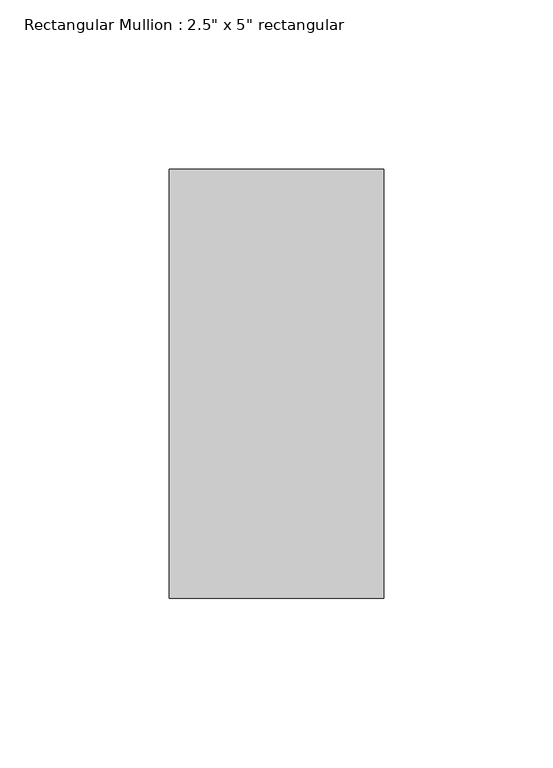
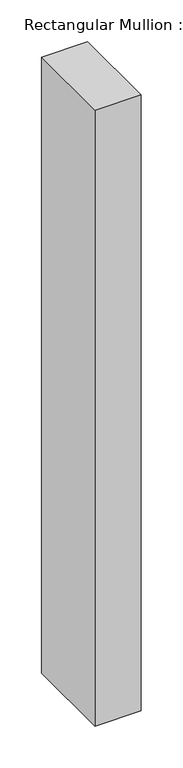
"""IFC4 building model written with IfcOpenShell, lengths in millimetres: member geometry."""

from ifc_helpers import new_model, si_unit, frame, origin, place, context, project, spatial, polyline, outline, extrude, source, transform, mapped, element, save


def member_06e32611(model_context):
    return source(origin(), model_context, "Body", "SweptSolid", [
        extrude(outline(polyline([(0.0, 63.5), (0.0, -63.5), (-63.5, -63.5), (-63.5, 63.5), (0.0, 63.5)])), frame((0.0, 0.0, -897.4039078), z_axis=(0.0, 0.0, 1.0), x_axis=(1.0, 0.0, 0.0)), (0.0, 0.0, 1.0), 897.4039078),
    ])


if __name__ == "__main__":
    model = new_model("IFC4")
    model_context = context("Model", 3, world=origin())
    ifc_project = project(units=[si_unit("LENGTHUNIT", "METRE", prefix="MILLI")], contexts=[model_context])
    site = spatial("IfcSite", under=ifc_project)
    building = spatial("IfcBuilding", under=site)
    placement = place(None, origin())
    member_shape = member_06e32611(model_context)
    element("IfcMember", 1, ObjectType="Rectangular Mullion : 2.5\" x 5\" rectangular", at=placement, inside=building, context=model_context, shape_type="MappedRepresentation", body=[
        mapped(member_shape, transform((0.0, 0.0, 0.0), x_axis=(1.0, 0.0, 0.0), y_axis=(0.0, 1.0, 0.0), z_axis=(0.0, 0.0, 1.0))),
    ])
    save(model, "model.ifc")

# Revit data of these elements
# Type "Rectangular Mullion : 2.5\" x 5\" rectangular"
#   built-in parameter 1007304 = 0.416667 (stored number, unit not read)
#   built-in parameter 1007301 = 0.104167 (stored number, unit not read)
#   built-in parameter 1007300 = 0.104167 (stored number, unit not read)
# Element 1 (IfcMember, "Rectangular Mullion : 2.5\" x 5\" rectangular")
#   Materials on its faces: "Aluminum"
# Materials
#   "Aluminum": class "Metal", colour RGB 247 247 247, transparency 0, Description = "Aluminum 6061", Cost = 0
